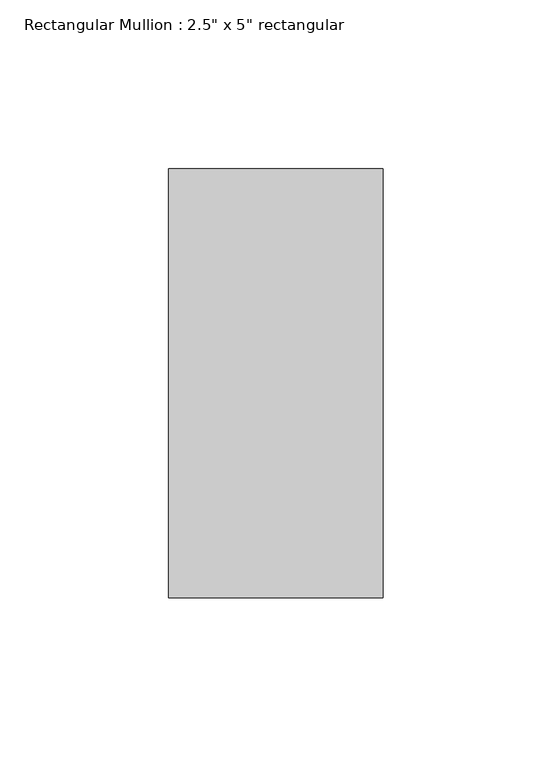
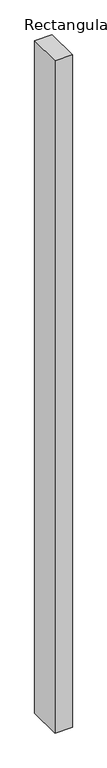
"""IFC4 building model written with IfcOpenShell, lengths in millimetres: member geometry."""

from ifc_helpers import new_model, si_unit, frame, origin, place, context, project, spatial, polyline, outline, extrude, source, transform, mapped, element, save


def member_4c337627(model_context):
    return source(origin(), model_context, "Body", "SweptSolid", [
        extrude(outline(polyline([(31.75, 63.5), (31.75, -63.5), (-31.75, -63.5), (-31.75, 63.5), (31.75, 63.5)])), frame((0.0, 0.0, -2581.7369027), z_axis=(0.0, 0.0, 1.0), x_axis=(1.0, 0.0, 0.0)), (0.0, 0.0, 1.0), 2581.7369027),
    ])


if __name__ == "__main__":
    model = new_model("IFC4")
    model_context = context("Model", 3, world=origin())
    ifc_project = project(units=[si_unit("LENGTHUNIT", "METRE", prefix="MILLI")], contexts=[model_context])
    site = spatial("IfcSite", under=ifc_project)
    building = spatial("IfcBuilding", under=site)
    placement = place(None, origin())
    member_shape = member_4c337627(model_context)
    element("IfcMember", 1, ObjectType="Rectangular Mullion : 2.5\" x 5\" rectangular", at=placement, inside=building, context=model_context, shape_type="MappedRepresentation", body=[
        mapped(member_shape, transform((0.0, 0.0, 0.0), x_axis=(1.0, 0.0, 0.0), y_axis=(0.0, 1.0, 0.0), z_axis=(0.0, 0.0, 1.0))),
    ])
    save(model, "model.ifc")

# Revit data of these elements
# Type "Rectangular Mullion : 2.5\" x 5\" rectangular"
#   built-in parameter 1007304 = 0.416667 (stored number, unit not read)
#   built-in parameter 1007301 = 0.104167 (stored number, unit not read)
#   built-in parameter 1007300 = 0.104167 (stored number, unit not read)
# Element 1 (IfcMember, "Rectangular Mullion : 2.5\" x 5\" rectangular")
#   Materials on its faces: "Gypsum Wall Board"
# Materials
#   "Gypsum Wall Board": class "Generic", colour RGB 127 127 127, transparency 0, Description = "Gypsum Wall Board", Cost = 0
